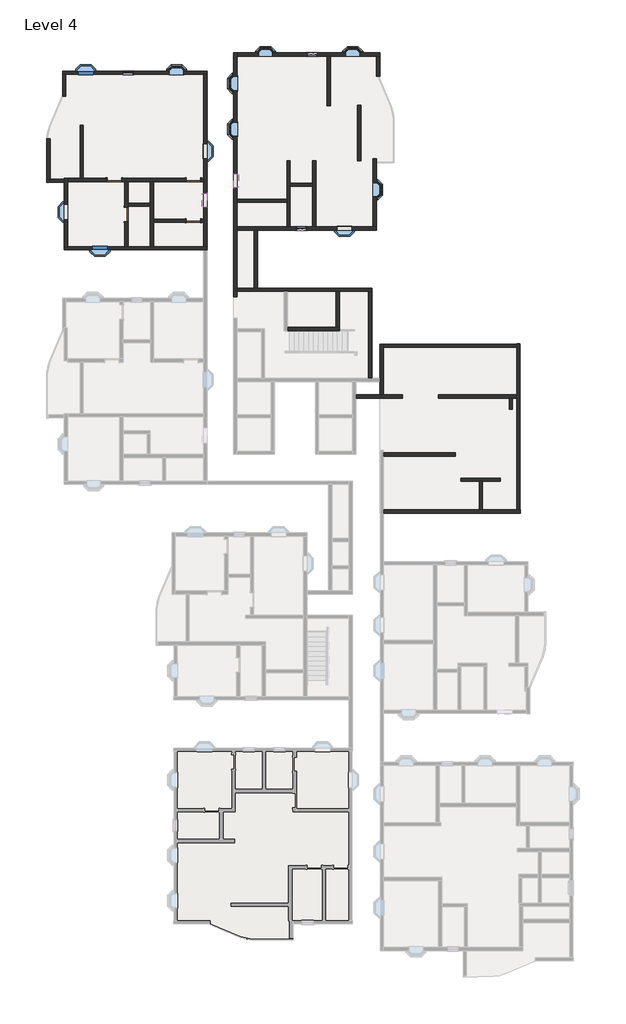
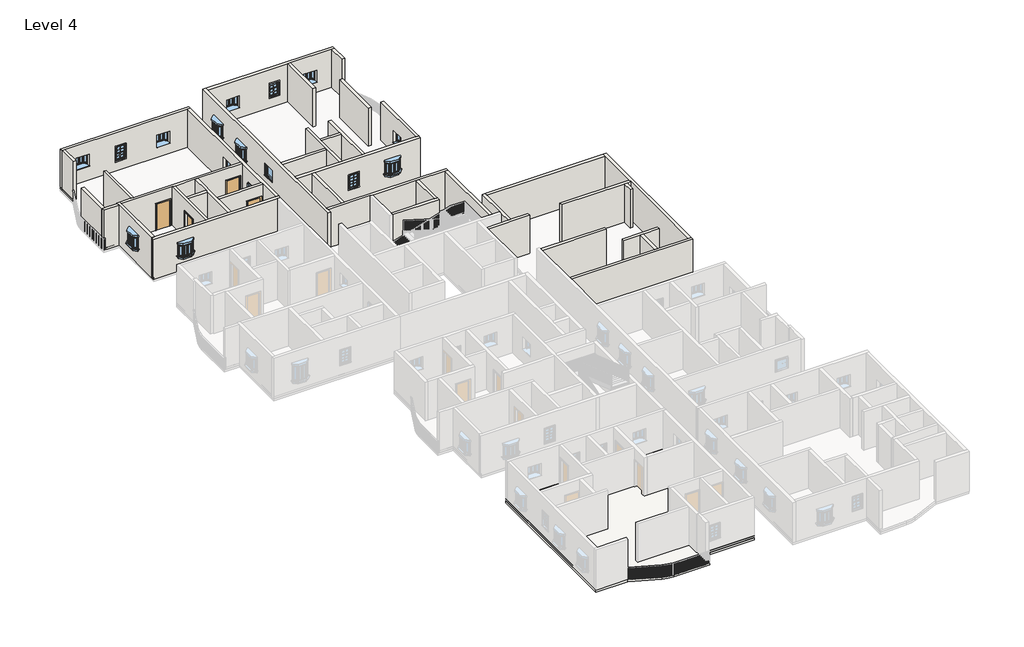
# One storey, part 4 of 14: 39 walls, 16 windows, 4 doors, 1 roof, 1 slab.
# Revit data of these elements (continued)
# Elements 31, 43 (IfcWall, "9\" w")
#   Top Offset = 0' - 0"
#   Base Offset = 0' - 0"
#   wall height = 10' - 0"
#   Phase Created = New Construction
#   Base Constraint = Level 4
#   Top Constraint = Level 5
#   Materials on its faces: "Default Wall", "Brick, Soldier Course"
# Element 32 (IfcWall, "9\" w")
#   Top Offset = 0' - 0"
#   Base Offset = 0' - 0"
#   wall height = 10' - 0"
#   Phase Created = New Construction
#   Base Constraint = Level 4
#   Top Constraint = Level 5
#   Materials on its faces: "Default Wall", "Brick, Soldier Course", "Earth"
# Element 33 (IfcWall, "9\" w")
#   Top Offset = 0' - 0"
#   Base Offset = 0' - 0"
#   wall height = 10' - 0"
#   Phase Created = New Construction
#   Base Constraint = Level 4
#   Top Constraint = Level 5
#   Materials on its faces: "Default Wall", "Earth"
# Elements 34, 35, 36 (IfcWall, "9\" w")
#   Top Offset = 0' - 0"
#   Base Offset = 0' - 0"
#   wall height = 10' - 0"
#   Phase Created = New Construction
#   Base Constraint = Level 4
#   Top Constraint = Level 5
#   Materials on its faces: "Default Wall", "Window Frame"
# Element 41 (IfcWall, "9\" w")
#   Top Offset = 0' - 0"
#   Base Offset = 0' - 0"
#   wall height = 10' - 0"
#   Phase Created = New Construction
#   Base Constraint = Level 4
#   Top Constraint = Level 5
#   Materials on its faces: "Default Wall", "Parking Stripe", "Default Mass Interior Wall"
# Element 42 (IfcWall, "9\" w")
#   Top Offset = 0' - 0"
#   Base Offset = 0' - 0"
#   wall height = 10' - 0"
#   Phase Created = New Construction
#   Base Constraint = Level 4
#   Top Constraint = Level 5
#   Materials on its faces: "Default Wall", "Parking Stripe", "Brick, Soldier Course"
# Element 44 (IfcWall, "9\" w")
#   Top Offset = 0' - 0"
#   Base Offset = 0' - 0"
#   wall height = 10' - 0"
#   Phase Created = New Construction
#   Base Constraint = Level 4
#   Top Constraint = Level 5
#   Materials on its faces: "Default Wall", "Parking Stripe"
# Element 45 (IfcWall, "9\" w")
#   Top Offset = 0' - 0"
#   Base Offset = 0' - 0"
#   wall height = 10' - 0"
#   Phase Created = New Construction
#   Base Constraint = Level 4
#   Top Constraint = Level 5
#   Materials on its faces: "Default Wall", "Grass"
# Element 46 (IfcWindow, "910x910mm")
#   Mark = "170"
#   Phase Created = New Construction
#   Materials on its faces: "Window Frame", "Glass"
# Element 47 (IfcWindow, "910x910mm")
#   Mark = "171"
#   Phase Created = New Construction
#   Materials on its faces: "Window Frame", "Glass"
# Element 48 (IfcWindow, "910x910mm")
#   Mark = "283"
#   Phase Created = New Construction
#   Materials on its faces: "Window Frame", "Glass"
# Element 49 (IfcWindow, "910x910mm")
#   Mark = "284"
#   Phase Created = New Construction
#   Materials on its faces: "Window Frame", "Glass"
# Element 50 (IfcWindow, "910x910mm")
#   Mark = "295"
#   Phase Created = New Construction
#   Materials on its faces: "Window Frame", "Glass"
# Element 51 (IfcWindow, "910x910mm")
#   Mark = "296"
#   Phase Created = New Construction
#   Materials on its faces: "Window Frame", "Glass"
# Element 52 (IfcWindow, "910x910mm")
#   Mark = "490"
#   Phase Created = New Construction
#   Materials on its faces: "Window Frame", "Glass"
# Element 53 (IfcWindow, "910x910mm")
#   Mark = "491"
#   Phase Created = New Construction
#   Materials on its faces: "Window Frame", "Glass"
# Element 54 (IfcWindow, "910x910mm")
#   Mark = "496"
#   Phase Created = New Construction
#   Materials on its faces: "Window Frame", "Glass"
# Element 55 (IfcWindow, "910x910mm")
#   Mark = "203"
#   Phase Created = New Construction
#   Materials on its faces: "Window Frame", "Glass"
# Element 56 (IfcWindow, "910x910mm")
#   Mark = "204"
#   Phase Created = New Construction
#   Materials on its faces: "Window Frame", "Glass"
# Element 57 (IfcWindow, "Window-Double-Hung : 26\" x 42\"")
#   Mark = "285"
#   Window Inset = 0' - 0"
#   Interior Wall Closure = 0' - 1 1/2"
#   Frame Extension = 0' - 1 1/4"
#   Exterior Wall Closure = 0' - 0 1/2"
#   Interior Trim Visibility = yes
#   Indicator Visibility = yes
#   Exterior Trim Visibility = yes
#   Phase Created = New Construction
#   Materials on its faces: "Wood - Stained", "Glass", "Clad - White"
# Element 58 (IfcWindow, "Window-Double-Hung : 26\" x 42\"")
#   Mark = "297"
#   Window Inset = 0' - 0"
#   Interior Wall Closure = 0' - 1 1/2"
#   Frame Extension = 0' - 1 1/4"
#   Exterior Wall Closure = 0' - 0 1/2"
#   Interior Trim Visibility = yes
#   Indicator Visibility = yes
#   Exterior Trim Visibility = yes
#   Phase Created = New Construction
#   Materials on its faces: "Wood - Stained", "Glass", "Clad - White"
# Element 59 (IfcWindow, "Window-Double-Hung : 26\" x 42\"")
#   Mark = "222"
#   Window Inset = 0' - 0"
#   Interior Wall Closure = 0' - 1 1/2"
#   Frame Extension = 0' - 1 1/4"
#   Exterior Wall Closure = 0' - 0 1/2"
#   Interior Trim Visibility = yes
#   Indicator Visibility = yes
#   Exterior Trim Visibility = yes
#   Phase Created = New Construction
#   Materials on its faces: "Wood - Stained", "Glass", "Clad - White"
# Element 60 (IfcWindow, "Windows_Sgl_w-Glazing_Bars : 910x910mm")
#   Mark = "492"
#   Phase Created = New Construction
#   Materials on its faces: "Window Frame", "Glass"
# Element 61 (IfcWindow, "Windows_Sgl_w-Glazing_Bars : 910x910mm")
#   Mark = "497"
#   Phase Created = New Construction
#   Materials on its faces: "Window Frame", "Glass"
# Materials
#   "Door - Panel": class "Wood", colour RGB 210 159 95, transparency 0, Cost = 0
#   "Door - Frame": colour RGB 118 70 51, transparency 0, Cost = 0
#   "Window Frame": colour RGB 249 249 249, transparency 0
#   "Glass": class "Glass", colour RGB 0 128 192, transparency 0.75, Description = "Soda Lime Glass", Cost = 0
#   "Wood - Stained": class "Wood", colour RGB 224 178 126, transparency 0, Cost = 0
#   "Clad - White": class "Wood", colour RGB 242 242 238, transparency 0, Cost = 0
#   "Default Roof": colour RGB 88 101 114, transparency 0, Cost = 0
#   "Default Floor": colour RGB 128 128 128, transparency 0, Cost = 0
#   "Default Wall": colour RGB 128 128 128, transparency 0, Cost = 0
#   "Parking Stripe": class "Paint", colour RGB 250 250 91, transparency 0, Cost = 0
#   "Carpet (1)": class "Carpet", colour RGB 124 80 67, transparency 0, Description = "Interior finish", Cost = 0
#   "Grass": class "Generic", colour RGB 104 137 66, transparency 0, Description = "Physical material.", Cost = 0
#   "Brick, Soldier Course": class "Masonry", colour RGB 170 98 104, transparency 0, Description = "Common brick soldier coursed", Cost = 0
#   "Default Mass Interior Wall": class "Generic", colour RGB 195 229 126, transparency 0, Cost = 0
#   "Earth": class "Generic", colour RGB 97 75 62, transparency 0, Description = "Soil", Cost = 0
